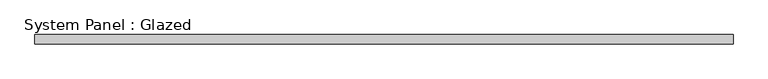
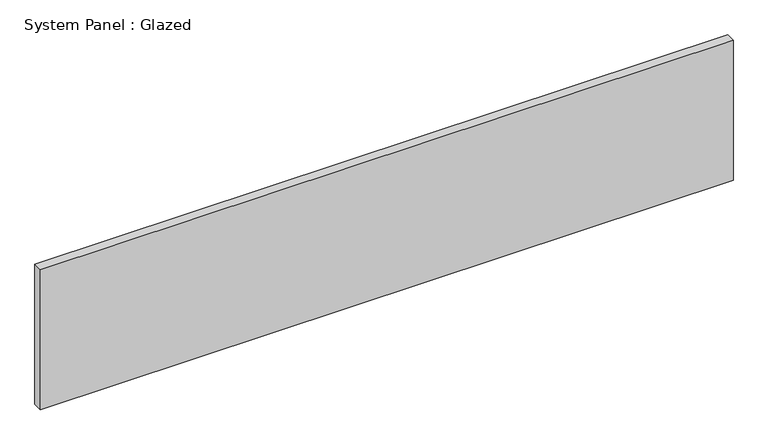
"""IFC4 building model written with IfcOpenShell, lengths in millimetres: plate geometry, System Panel : Glazed."""

from ifc_helpers import new_model, si_unit, origin, origin_with_axes, place, context, project, spatial, polyline, outline, extrude, source, transform, mapped, element, save


def system_panel_glazed_db63c8d7(model_context):
    return source(origin(), model_context, "Body", "SweptSolid", [
        extrude(outline(polyline([(950.7907705, 19.05), (-950.7907705, 19.05), (-950.7907705, 44.45), (950.7907705, 44.45), (950.7907705, 19.05)])), origin_with_axes(), (0.0, 0.0, 1.0), 406.4342224),
    ])


if __name__ == "__main__":
    model = new_model("IFC4")
    model_context = context("Model", 3, world=origin())
    ifc_project = project(units=[si_unit("LENGTHUNIT", "METRE", prefix="MILLI")], contexts=[model_context])
    site = spatial("IfcSite", under=ifc_project)
    building = spatial("IfcBuilding", under=site)
    placement = place(None, origin())
    system_panel_glazed_shape = system_panel_glazed_db63c8d7(model_context)
    element("IfcPlate", 1, ObjectType="System Panel : Glazed", at=placement, inside=building, context=model_context, shape_type="MappedRepresentation", body=[
        mapped(system_panel_glazed_shape, transform((0.0, 0.0, 0.0), x_axis=(1.0, 0.0, 0.0), y_axis=(0.0, 1.0, 0.0), z_axis=(0.0, 0.0, 1.0))),
    ])
    save(model, "model.ifc")

# Revit data of these elements
# Type "System Panel : Glazed"
#   Construction Type Id = "GSP4R"
#   Analytic Construction = "1/8 in Pilkington single glazing"
#   Visual Light Transmittance = 0.9
#   Solar Heat Gain Coefficient = 0.86
#   Heat Transfer Coefficient (U) = 1.18115 BTU/(h·ft²·°F)
#   Define Thermal Properties by = 1
# Element 1 (IfcPlate, "System Panel : Glazed")
#   Materials on its faces: "Glass"
# Materials
#   "Glass": class "Glass", colour RGB 0 128 192, transparency 0.75, Description = "Soda Lime Glass", Cost = 0
